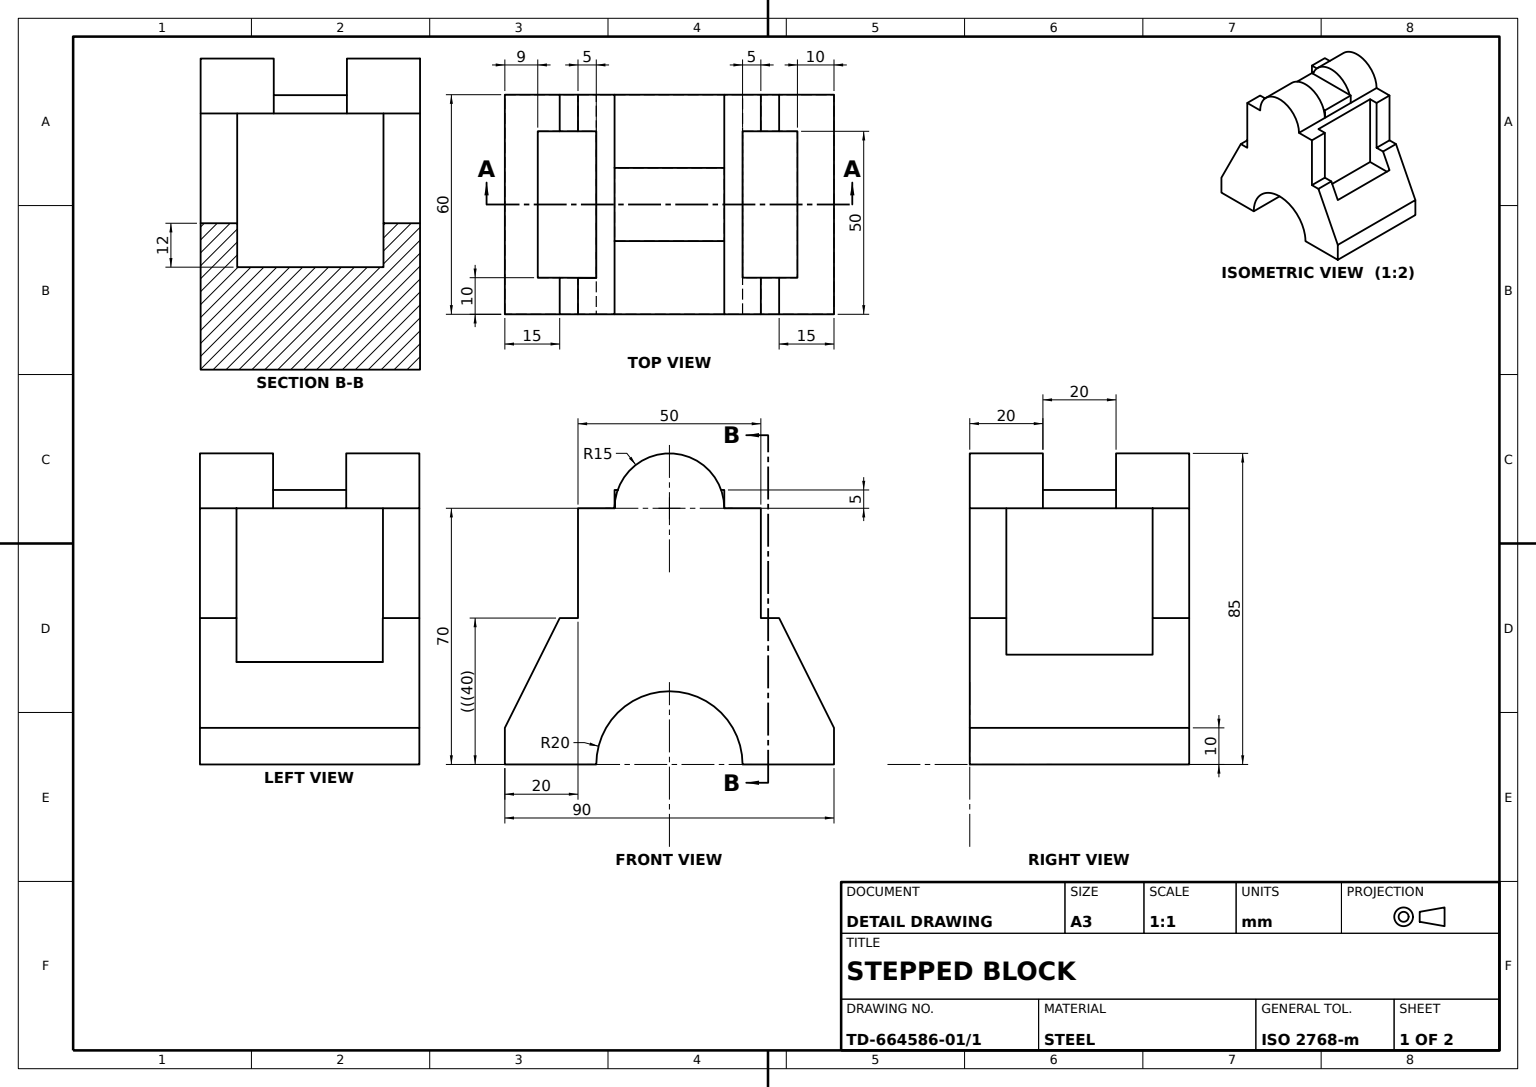
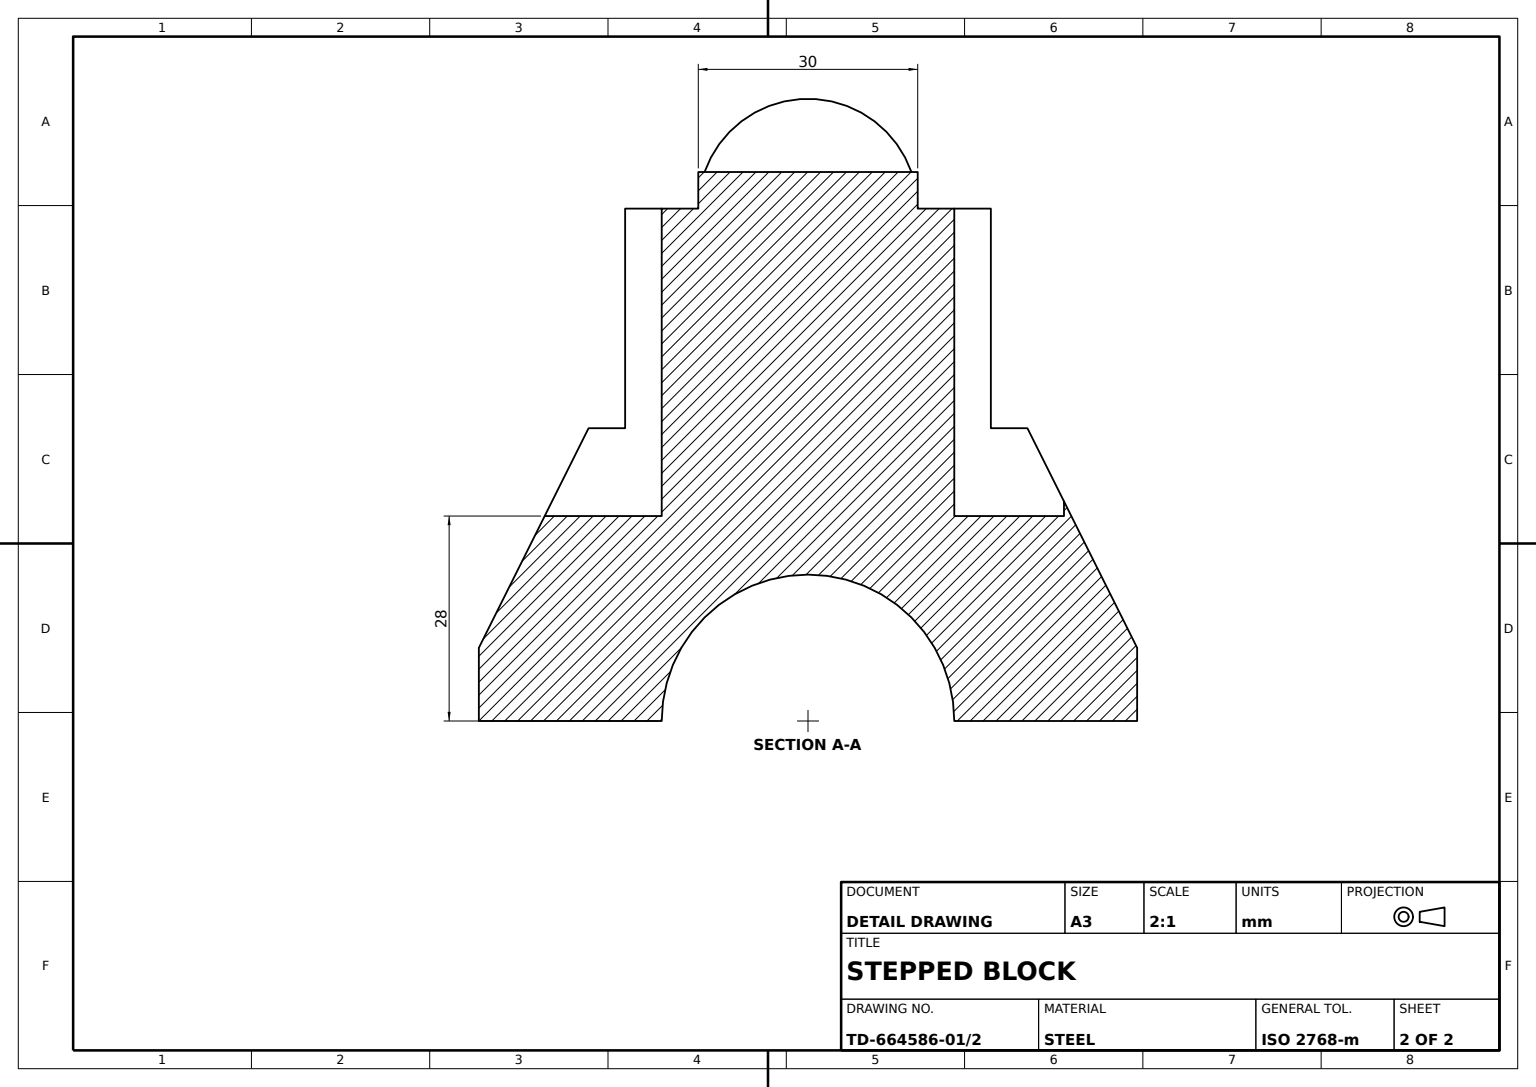
SolidWorks part; units mm, degrees
material "Plain Carbon Steel"
ref_plane "Front Plane" through (0, 0, 0) normal (0, 0, 1) x (1, 0, 0)
ref_plane "Top Plane" through (0, 0, 0) normal (0, 1, 0) x (1, 0, 0)
ref_plane "Right Plane" through (0, 0, 0) normal (1, 0, 0) x (0, 0, -1)
sketch "Arched Body Profile Sketch" plane through (0, 0, 0) normal (0, 0, 1) x (1, 0, 0)
  line L0 (0, 0) -> (25, 0)
  line L1 (90, 0) -> (90, 10)
  line L5 (0, 0) -> (0, 10)
  line L6 (65, 0) -> (90, 0)
  line L7 (20, 40) -> (15, 40)
  line L8 (15, 40) -> (0, 10)
  line L9 (70, 40) -> (75, 40)
  line L10 (75, 40) -> (90, 10)
  line L11 (30, 70) -> (20, 70)
  line L12 (20, 70) -> (20, 40)
  line L13 (60, 70) -> (70, 70)
  line L14 (70, 70) -> (70, 40)
  arc A0 (65, 0) -> (25, 0) centre (45, 0) ccw
  arc A1 (60, 70) -> (30, 70) centre (45, 70) ccw
  dimension "D1" = 20
  dimension "D2" = 15
  dimension "D3" = 15
  dimension "D4" = 20
  dimension "D5" = 45
  dimension "D6" = 40
extrude "Arched Body 60" add sketch "Arched Body Profile Sketch" along normal blind 60
sketch "Pocket A Step Sketch" plane through (20, 0, 0) normal (-1, 0, 0) x (0, 0, 1)
  line L0 (30, 70) -> (10, 70)
  line L1 (60, 70) -> (0, 70) construction
  line L2 (10, 70) -> (10, 40)
  line L3 (60, 40) -> (0, 40) construction
  line L4 (10, 40) -> (50.0469, 40)
  line L5 (60, 40) -> (0, 40) construction
  line L6 (50.0469, 40) -> (50.0469, 70)
  line L7 (50.0469, 70) -> (30, 70)
  line L8 (0, 70) -> (0, 40) construction
  dimension "D1" = 10
  dimension "D2" = 50.0469
extrude "Pocket A Step Cut 5" cut sketch "Pocket A Step Sketch" against normal blind 5
sketch "Pocket A Sketch" plane through (0, 40, 0) normal (0, 1, 0) x (1, 0, 0)
  line L0 (20, -10) -> (15, -10)
  line L1 (15, -60) -> (15, 0) construction
  line L3 (15, -50) -> (25, -50.0469)
  line L4 (25, -50.0469) -> (25, -10)
  line L5 (25, -10) -> (20, -10)
  line L6 (15, -10) -> (5, -10)
  line L7 (5, -10) -> (5, -50)
  line L8 (5, -50) -> (15, -50)
  line L9 (20, -60) -> (15, -60) construction
  dimension "D1" = 10
  dimension "D2" = 10
extrude "Pocket A Cut 12" cut sketch "Pocket A Sketch" against normal blind 12
sketch "Pocket B Step Sketch" plane through (70, 0, 0) normal (1, 0, 0) x (0, 0, -1)
  line L0 (-30, 70) -> (-50, 70)
  line L1 (-60, 70) -> (0, 70) construction
  line L2 (-60, 70) -> (0, 70) construction
  line L3 (-50, 70) -> (-50, 40)
  line L4 (-60, 40) -> (0, 40) construction
  line L5 (-50, 40) -> (-10, 40)
  line L6 (-60, 40) -> (0, 40) construction
  line L7 (-10, 40) -> (-10, 70)
  line L8 (-10, 70) -> (-30, 70)
  line L9 (0, 40) -> (0, 70) construction
  dimension "D1" = 10
extrude "Pocket B Step Cut 5" cut sketch "Pocket B Step Sketch" against normal blind 5
sketch "Pocket B Sketch" plane through (0, 40, 0) normal (0, 1, 0) x (1, 0, 0)
  line L0 (65, -10) -> (80, -10)
  line L1 (80, -10) -> (80, -50)
  line L2 (80, -50) -> (65, -50)
  line L3 (65, -50) -> (65, -10)
  line L4 (65, -50) -> (65, -10) construction
  dimension "D1" = 15
extrude "Pocket B Cut 12" cut sketch "Pocket B Sketch" against normal blind 12
sketch "Top Half-Round Cut Sketch" plane through (0, 0, 0) normal (0, 0, -1) x (-1, 0, 0)
  line L0 (-60, 70) -> (-30, 70)
  arc A0 (-30, 70) -> (-60, 70) centre (-45, 70) ccw
extrude "Top Half-Round Cut 40" cut sketch "Top Half-Round Cut Sketch" against normal blind 40
sketch "Top Pad Sketch" plane through (0, 70, 0) normal (0, 1, 0) x (1, 0, 0)
  line L0 (30, -40) -> (30, -20)
  line L1 (30, -20) -> (60, -20)
  line L2 (60, -20) -> (60, -40)
  line L3 (60, -40) -> (30, -40)
  line L5 (30, -60) -> (20, -60) construction
  dimension "D1" = 40
extrude "Top Pad 5" add sketch "Top Pad Sketch" along normal blind 5
sketch "Top Half-Round Boss Sketch" plane through (0, 0, 0) normal (0, 0, -1) x (-1, 0, 0)
  line L0 (-60, 70) -> (-30, 70)
  line L1 (-30, 75) -> (-30, 70) construction
  line L2 (-60, 70) -> (-30, 70) construction
  arc A0 (-30, 70) -> (-60, 70) centre (-45, 70) ccw
extrude "Top Half-Round Boss 20" add sketch "Top Half-Round Boss Sketch" against normal blind 20
